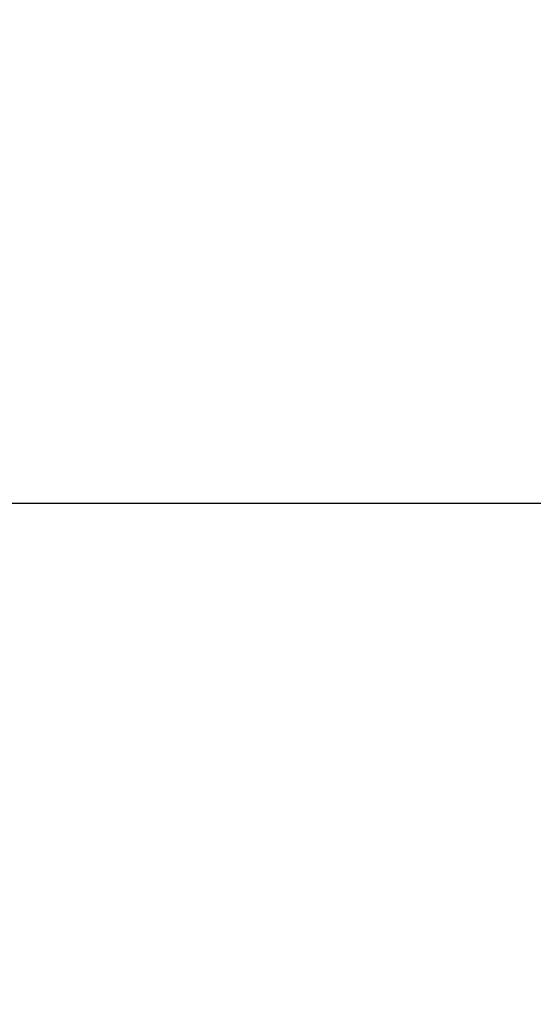
# Model space of a CAD drawing. Units: inches. Extents: x 2083 to 3317, y 1141 to 2115.
# Tile 237 of 256: x 3128.28 to 3136.89, y 1254.86 to 1271.37. Entities that reach past the tile are written whole.
import ezdxf

# ---------------------------------------------------------------- set-up
doc = ezdxf.new("R2010")
doc.units = ezdxf.units.IN
doc.layers.add('A-ANNO-DIMS', color=2, linetype='Continuous', lineweight=18)
doc.styles.get("Standard").update_dxf_attribs({"font": 'arial.ttf'})
doc.dimstyles.new('ISO-25', dxfattribs={"dimtxt": 12, "dimasz": 12, "dimexe": 1.25, "dimexo": 0.625, "dimtad": 1, "dimlunit": 3, "dimtxsty": 'Standard', "dimcen": 2.5, "dimadec": 0, "dimazin": 0, "dimtfac": 1, "dimtmove": 0, "dimatfit": 3, "dimfxl": 1, "dimarcsym": 0})

# ---------------------------------------------------------------- blocks, each defined once
blk = doc.blocks.new('*D9')
at = {"layer": 'A-ANNO-DIMS', "color": 0, "lineweight": -2, "transparency": 16777216}
for p, q in [((3127.585, 1486.761), (3190.403, 1486.761)), ((3189.153, 1474.761), (3189.153, 1275.261)), ((3127.585, 1263.261), (3190.403, 1263.261))]:
    blk.add_line(p, q, dxfattribs=at)
at = {"layer": 'A-ANNO-DIMS', "color": 0, "transparency": 16777216}
for points in [[(3187.153, 1474.761), (3191.153, 1474.761), (3189.153, 1486.761)], [(3187.153, 1275.261), (3191.153, 1275.261), (3189.153, 1263.261)]]:
    blk.add_solid(points, dxfattribs=at)
at = {"layer": 'Defpoints', "color": 0, "transparency": 16777216}
for p in [(3126.96, 1486.761), (3126.96, 1263.261), (3189.153, 1263.261)]:
    blk.add_point(p, dxfattribs=at)
at = {"layer": 'A-ANNO-DIMS', "color": 0, "transparency": 16777216, "insert": (3182.401, 1375.011), "char_height": 12, "attachment_point": 5, "rotation": 90}
blk.add_mtext('18\'-7.5"', dxfattribs=at)
blk = doc.blocks.new('*D26')
at = {"layer": 'A-ANNO-DIMS', "color": 0, "lineweight": -2, "transparency": 16777216}
for p, q in [((3088.986, 1274.915), (3088.986, 1270.952)), ((3111.24, 1274.915), (3111.24, 1270.952)), ((3076.986, 1272.202), (2840.262, 1272.202)), ((3111.24, 1272.202), (3088.986, 1272.202)), ((3123.24, 1272.202), (3135.24, 1272.202))]:
    blk.add_line(p, q, dxfattribs=at)
at = {"layer": 'A-ANNO-DIMS', "color": 0, "transparency": 16777216}
for points in [[(3076.986, 1274.202), (3076.986, 1270.202), (3088.986, 1272.202)], [(3123.24, 1274.202), (3123.24, 1270.202), (3111.24, 1272.202)]]:
    blk.add_solid(points, dxfattribs=at)
at = {"layer": 'Defpoints', "color": 0, "transparency": 16777216}
for p in [(3088.986, 1275.54), (3111.24, 1275.54), (3088.986, 1272.202)]:
    blk.add_point(p, dxfattribs=at)
at = {"layer": 'A-ANNO-DIMS', "color": 0, "transparency": 16777216, "insert": (2952.624, 1279.032), "char_height": 12, "attachment_point": 5}
blk.add_mtext('NIGHTSTAND 1\'-10 1/2" TYP.', dxfattribs=at)
blk = doc.blocks.new('*D27')
at = {"layer": 'A-ANNO-DIMS', "color": 0, "lineweight": -2, "transparency": 16777216}
for p, q in [((3114.578, 1309.794), (3114.578, 1321.794)), ((3111.865, 1297.794), (3115.828, 1297.794)), ((3114.578, 1297.794), (3114.578, 1275.54)), ((3111.865, 1275.54), (3115.828, 1275.54)), ((3114.578, 1263.54), (3114.578, 1140.989))]:
    blk.add_line(p, q, dxfattribs=at)
at = {"layer": 'A-ANNO-DIMS', "color": 0, "transparency": 16777216}
for points in [[(3112.578, 1309.794), (3116.578, 1309.794), (3114.578, 1297.794)], [(3112.578, 1263.54), (3116.578, 1263.54), (3114.578, 1275.54)]]:
    blk.add_solid(points, dxfattribs=at)
at = {"layer": 'Defpoints', "color": 0, "transparency": 16777216}
for p in [(3111.24, 1297.794), (3111.24, 1275.54), (3114.578, 1275.54)]:
    blk.add_point(p, dxfattribs=at)
at = {"layer": 'A-ANNO-DIMS', "color": 0, "transparency": 16777216, "insert": (3107.749, 1196.264), "char_height": 12, "attachment_point": 5, "rotation": 90}
blk.add_mtext('1\'-10 1/2" TYP.', dxfattribs=at)
blk = doc.blocks.new('*D35')
at = {"layer": 'A-ANNO-DIMS', "color": 0, "lineweight": -2, "transparency": 16777216}
for p, q in [((3127.585, 2020.761), (3180.56, 2020.761)), ((3179.31, 1275.261), (3179.31, 2008.761)), ((3127.585, 1263.261), (3180.56, 1263.261))]:
    blk.add_line(p, q, dxfattribs=at)
at = {"layer": 'A-ANNO-DIMS', "color": 0, "transparency": 16777216}
for points in [[(3177.31, 2008.761), (3181.31, 2008.761), (3179.31, 2020.761)], [(3177.31, 1275.261), (3181.31, 1275.261), (3179.31, 1263.261)]]:
    blk.add_solid(points, dxfattribs=at)
at = {"layer": 'Defpoints', "color": 0, "transparency": 16777216}
for p in [(3126.96, 2020.761), (3179.31, 2020.761), (3126.96, 1263.261)]:
    blk.add_point(p, dxfattribs=at)
at = {"layer": 'A-ANNO-DIMS', "color": 0, "transparency": 16777216, "insert": (3172.476, 1642.011), "char_height": 12, "attachment_point": 5, "rotation": 90}
blk.add_mtext('63\'-1 1/2"', dxfattribs=at)

msp = doc.modelspace()

# ---------------------------------------------------------------- dimensions: what is measured, and where the dimension line sits
at = {"layer": 'A-ANNO-DIMS'}
for base, p1, p2, override, picture, middle in [((3179.31, 2020.761), (3126.96, 1263.261), (3126.96, 2020.761), {"dimdec": 1, "dimlfac": 1, "dimrnd": 0, "dimzin": 1, "dimdsep": 46, "dimlunit": 4, "dimfrac": 2}, '*D35', (3172.476, 1642.011)), ((3189.153, 1263.261), (3126.96, 1486.761), (3126.96, 1263.261), {"dimclrd": 0, "dimclre": 0, "dimclrt": 0}, '*D9', (3182.401, 1375.011))]:
    dim = msp.add_linear_dim(base=base, p1=p1, p2=p2, angle=90, dimstyle='ISO-25', override=override, dxfattribs=at)
    dim.commit()
    dim.dimension.update_dxf_attribs({"geometry": picture, "text_midpoint": middle})
for base, p1, p2, angle, text, picture, middle in [((3114.578, 1275.54), (3111.24, 1297.794), (3111.24, 1275.54), 270, '<> TYP.', '*D27', (3107.749, 1196.264)), ((3088.986, 1272.202), (3111.24, 1275.54), (3088.986, 1275.54), 180, 'NIGHTSTAND <> TYP.', '*D26', (2952.624, 1279.032))]:
    dim = msp.add_linear_dim(base=base, p1=p1, p2=p2, angle=angle, text=text, dimstyle='ISO-25', override={"dimdec": 1, "dimlfac": 1, "dimrnd": 0, "dimzin": 1, "dimdsep": 46, "dimlunit": 4, "dimfrac": 2}, dxfattribs=at)
    dim.commit()
    dim.dimension.update_dxf_attribs({"geometry": picture, "text_midpoint": middle})

doc.saveas('drawing.dxf')
